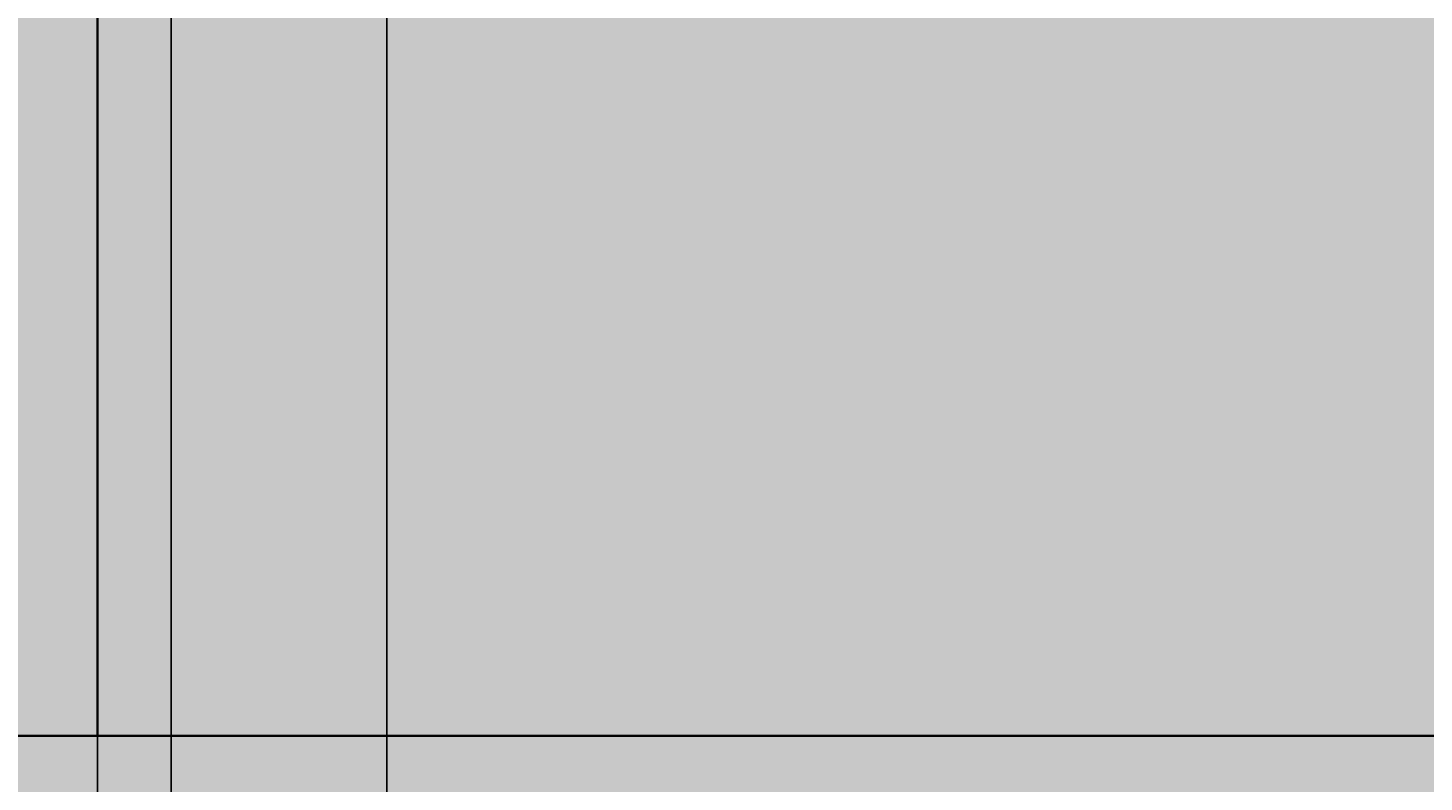
# Model space of a CAD drawing. Units: feet. Extents: x 2695 to 2912, y 795 to 1139.
# Tile 68 of 83: x 2769 to 2805, y 1062 to 1081. Entities that reach past the tile are written whole.
import ezdxf

# ---------------------------------------------------------------- set-up
doc = ezdxf.new("R2010")
doc.units = ezdxf.units.FT
for name, color, linetype, lineweight in [('A-ANNO-DIMS', 2, 'Continuous', 18), ('A-ELEV', 7, 'Continuous', 35), ('A-ELEV-PATT', 252, 'Continuous', 13)]:
    doc.layers.add(name, color=color, linetype=linetype, lineweight=lineweight)
doc.styles.get("Standard").update_dxf_attribs({"font": 'arial.ttf'})
doc.dimstyles.get("Standard").update_dxf_attribs({"dimtxt": 0.18, "dimasz": 0.18, "dimexe": 0.18, "dimexo": 0.0625, "dimgap": 0.09, "dimtad": 0, "dimtih": 1, "dimtoh": 1, "dimdec": 1, "dimzin": 0, "dimdsep": 46, "dimlunit": 3, "dimtxsty": 'Standard', "dimcen": 0.09, "dimadec": 0, "dimazin": 0, "dimtfac": 1, "dimtdec": 1, "dimtofl": 0, "dimtmove": 0, "dimatfit": 3, "dimfxl": 1, "dimtolj": 1, "dimtzin": 0, "dimarcsym": 0})

# ---------------------------------------------------------------- blocks, each defined once
blk = doc.blocks.new('*D8')
at = {"layer": 'A-ANNO-DIMS', "color": 0, "lineweight": -2, "transparency": 16777216}
for p, q in [((2715.885, 1050.373), (2715.885, 1138.886)), ((2716.065, 1138.706), (2742.866, 1138.706)), ((2770.456, 1138.706), (2743.655, 1138.706)), ((2770.636, 1122.993), (2770.636, 1138.886))]:
    blk.add_line(p, q, dxfattribs=at)
at = {"layer": 'A-ANNO-DIMS', "color": 0, "transparency": 16777216}
for points in [[(2716.065, 1138.736), (2716.065, 1138.676), (2715.885, 1138.706)], [(2770.456, 1138.736), (2770.456, 1138.676), (2770.636, 1138.706)]]:
    blk.add_solid(points, dxfattribs=at)
at = {"layer": 'Defpoints', "color": 0, "transparency": 16777216}
for p in [(2770.636, 1138.706), (2770.636, 1122.931), (2715.885, 1050.311)]:
    blk.add_point(p, dxfattribs=at)
at = {"layer": 'A-ANNO-DIMS', "color": 0, "transparency": 16777216, "insert": (2743.261, 1138.706), "char_height": 0.18, "attachment_point": 5}
blk.add_mtext('\\A1;54.75', dxfattribs=at)
blk = doc.blocks.new('*D9')
at = {"layer": 'A-ANNO-DIMS', "color": 0, "lineweight": -2, "transparency": 16777216}
for p, q in [((2770.636, 1122.993), (2770.636, 1138.886)), ((2770.816, 1138.706), (2773.942, 1138.706)), ((2777.854, 1138.706), (2774.728, 1138.706)), ((2778.034, 1020.886), (2778.034, 1138.886))]:
    blk.add_line(p, q, dxfattribs=at)
at = {"layer": 'A-ANNO-DIMS', "color": 0, "transparency": 16777216}
for points in [[(2770.816, 1138.736), (2770.816, 1138.676), (2770.636, 1138.706)], [(2777.854, 1138.736), (2777.854, 1138.676), (2778.034, 1138.706)]]:
    blk.add_solid(points, dxfattribs=at)
at = {"layer": 'Defpoints', "color": 0, "transparency": 16777216}
for p in [(2778.034, 1138.706), (2770.636, 1122.931), (2778.034, 1020.824)]:
    blk.add_point(p, dxfattribs=at)
at = {"layer": 'A-ANNO-DIMS', "color": 0, "transparency": 16777216, "insert": (2774.335, 1138.706), "char_height": 0.18, "attachment_point": 5}
blk.add_mtext('\\A1;7.398', dxfattribs=at)
blk = doc.blocks.new('*D10')
at = {"layer": 'A-ANNO-DIMS', "color": 0, "lineweight": -2, "transparency": 16777216}
for p, q in [((2778.034, 1020.886), (2778.034, 1138.886)), ((2778.214, 1138.706), (2810.411, 1138.706)), ((2843.395, 1138.706), (2811.198, 1138.706)), ((2843.575, 1020.886), (2843.575, 1138.886))]:
    blk.add_line(p, q, dxfattribs=at)
at = {"layer": 'A-ANNO-DIMS', "color": 0, "transparency": 16777216}
for points in [[(2778.214, 1138.736), (2778.214, 1138.676), (2778.034, 1138.706)], [(2843.395, 1138.736), (2843.395, 1138.676), (2843.575, 1138.706)]]:
    blk.add_solid(points, dxfattribs=at)
at = {"layer": 'Defpoints', "color": 0, "transparency": 16777216}
for p in [(2843.575, 1138.706), (2778.034, 1020.824), (2843.575, 1020.824)]:
    blk.add_point(p, dxfattribs=at)
at = {"layer": 'A-ANNO-DIMS', "color": 0, "transparency": 16777216, "insert": (2810.805, 1138.706), "char_height": 0.18, "attachment_point": 5}
blk.add_mtext('\\A1;65.54', dxfattribs=at)
blk = doc.blocks.new('*D48')
at = {"layer": 'A-ANNO-DIMS', "color": 0, "lineweight": -2, "transparency": 16777216}
for p, q in [((2770.636, 972.03), (2770.636, 1138.886)), ((2770.816, 1138.706), (2771.263, 1138.706)), ((2772.342, 1138.706), (2771.894, 1138.706)), ((2772.522, 972.03), (2772.522, 1138.886))]:
    blk.add_line(p, q, dxfattribs=at)
at = {"layer": 'A-ANNO-DIMS', "color": 0, "transparency": 16777216}
for points in [[(2770.816, 1138.736), (2770.816, 1138.676), (2770.636, 1138.706)], [(2772.342, 1138.736), (2772.342, 1138.676), (2772.522, 1138.706)]]:
    blk.add_solid(points, dxfattribs=at)
at = {"layer": 'Defpoints', "color": 0, "transparency": 16777216}
for p in [(2772.522, 1138.706), (2770.636, 971.967), (2772.522, 971.967)]:
    blk.add_point(p, dxfattribs=at)
at = {"layer": 'A-ANNO-DIMS', "color": 0, "transparency": 16777216, "insert": (2771.579, 1138.706), "char_height": 0.18, "attachment_point": 5}
blk.add_mtext('\\A1;1.89', dxfattribs=at)
blk = doc.blocks.new('*D49')
at = {"layer": 'A-ANNO-DIMS', "color": 0, "lineweight": -2, "transparency": 16777216}
for p, q in [((2772.522, 972.03), (2772.522, 1138.886)), ((2772.702, 1138.706), (2790.888, 1138.706)), ((2809.861, 1138.706), (2791.674, 1138.706)), ((2810.041, 972.03), (2810.041, 1138.886))]:
    blk.add_line(p, q, dxfattribs=at)
at = {"layer": 'A-ANNO-DIMS', "color": 0, "transparency": 16777216}
for points in [[(2772.702, 1138.736), (2772.702, 1138.676), (2772.522, 1138.706)], [(2809.861, 1138.736), (2809.861, 1138.676), (2810.041, 1138.706)]]:
    blk.add_solid(points, dxfattribs=at)
at = {"layer": 'Defpoints', "color": 0, "transparency": 16777216}
for p in [(2810.041, 1138.706), (2772.522, 971.967), (2810.041, 971.967)]:
    blk.add_point(p, dxfattribs=at)
at = {"layer": 'A-ANNO-DIMS', "color": 0, "transparency": 16777216, "insert": (2791.281, 1138.706), "char_height": 0.18, "attachment_point": 5}
blk.add_mtext('\\A1;37.52', dxfattribs=at)

msp = doc.modelspace()

# ---------------------------------------------------------------- hatches: boundary and pattern name
at = {"layer": 'A-ELEV-PATT'}
h = msp.add_hatch(color=256, dxfattribs=at)
h.set_gradient(color1=(255, 255, 255), tint=1)
h.paths.add_polyline_path([(2770.6361, 1122.9306), (2710.6361, 1122.9306), (2710.6361, 1118.4096), (2770.6361, 1118.4096)])
h.paths.add_polyline_path([(2890.6361, 1107.8588), (2770.6361, 1107.8588), (2770.6361, 1103.3378), (2890.6361, 1103.3378)])
h.paths.add_polyline_path([(2890.6361, 1062.9306), (2710.6361, 1062.9306), (2710.6361, 1056.9306), (2710.6361, 936.9306), (2710.6361, 924.3105), (2716.5358, 924.3105), (2890.6361, 924.3105), (2890.6361, 936.9306), (2715.8852, 936.9306), (2715.8852, 1050.3105), (2890.6361, 1050.3105)])
h.paths.add_polyline_path([(2716.5358, 924.3105), (2710.6361, 924.3105), (2710.6361, 810.9306), (2716.5358, 810.9306)])
h = msp.add_hatch(color=256, dxfattribs=at)
h.set_gradient(color1=(147, 149, 152), color2=(147, 149, 152), tint=1)
h.paths.add_polyline_path([(2770.6361, 1118.4096), (2710.6361, 1118.4096), (2710.6361, 1062.9306), (2770.6361, 1062.9306)])
h.paths.add_polyline_path([(2890.6361, 1103.3378), (2770.6361, 1103.3378), (2770.6361, 1062.9306), (2890.6361, 1062.9306)])
h.paths.add_polyline_path([(2730.7081, 1048.1052), (2755.1125, 1048.1052), (2755.1125, 936.9306), (2770.6361, 936.9306), (2770.6361, 1050.3105), (2715.8852, 1050.3105), (2715.8852, 936.9306), (2730.7081, 936.9306)])
h.paths.add_polyline_path([(2890.6361, 1050.3105), (2770.6361, 1050.3105), (2770.6361, 971.9673), (2778.0341, 971.9673), (2778.0341, 1020.8235), (2843.575, 1020.8235), (2843.575, 971.9673), (2890.6361, 971.9673)])
h.paths.add_polyline_path([(2888.1882, 970.7156), (2843.575, 970.7156), (2843.575, 964.8267), (2888.1882, 964.8267)])
h.paths.add_polyline_path([(2888.1882, 964.1328), (2843.575, 964.1328), (2843.575, 956.614), (2888.1882, 956.614)])
h.paths.add_polyline_path([(2888.1882, 955.9202), (2843.575, 955.9202), (2843.575, 949.2892), (2888.1882, 949.2892)])
h.paths.add_polyline_path([(2888.1882, 948.5954), (2843.575, 948.5954), (2843.575, 941.3507), (2888.1882, 941.3507)])
h.paths.add_polyline_path([(2888.1882, 940.6569), (2843.575, 940.6569), (2843.575, 936.9306), (2888.1882, 936.9306)])
h.paths.add_polyline_path([(2890.6361, 970.7156), (2888.9368, 970.7156), (2888.9368, 964.8267), (2890.6361, 964.8267)])
h.paths.add_polyline_path([(2890.6361, 964.1328), (2888.9368, 964.1328), (2888.9368, 956.614), (2890.6361, 956.614)])
h.paths.add_polyline_path([(2890.6361, 955.9202), (2888.9368, 955.9202), (2888.9368, 949.2892), (2890.6361, 949.2892)])
h.paths.add_polyline_path([(2890.6361, 940.6569), (2888.9368, 940.6569), (2888.9368, 936.9306), (2890.6361, 936.9306)])
h.paths.add_polyline_path([(2890.6361, 948.5954), (2888.9368, 948.5954), (2888.9368, 941.3507), (2890.6361, 941.3507)])
h.paths.add_polyline_path([(2772.5216, 970.7156), (2770.6361, 970.7156), (2770.6361, 964.8267), (2772.5216, 964.8267)])
h.paths.add_polyline_path([(2772.5216, 964.1328), (2770.6361, 964.1328), (2770.6361, 956.614), (2772.5216, 956.614)])
h.paths.add_polyline_path([(2772.5216, 955.9202), (2770.6361, 955.9202), (2770.6361, 949.2892), (2772.5216, 949.2892)])
h.paths.add_polyline_path([(2772.5216, 948.5954), (2770.6361, 948.5954), (2770.6361, 941.3507), (2772.5216, 941.3507)])
h.paths.add_polyline_path([(2772.5216, 940.6569), (2770.6361, 940.6569), (2770.6361, 936.9306), (2772.5216, 936.9306)])
h.paths.add_polyline_path([(2778.0341, 940.6569), (2773.2702, 940.6569), (2773.2702, 936.9306), (2778.0341, 936.9306)])
h.paths.add_polyline_path([(2778.0341, 970.7156), (2773.2702, 970.7156), (2773.2702, 964.8267), (2778.0341, 964.8267)])
h.paths.add_polyline_path([(2778.0341, 964.1328), (2773.2702, 964.1328), (2773.2702, 956.614), (2778.0341, 956.614)])
h.paths.add_polyline_path([(2778.0341, 955.9202), (2773.2702, 955.9202), (2773.2702, 949.2892), (2778.0341, 949.2892)])
h.paths.add_polyline_path([(2778.0341, 948.5954), (2773.2702, 948.5954), (2773.2702, 941.3507), (2778.0341, 941.3507)])
h.paths.add_polyline_path([(2810.0407, 940.6569), (2780.0341, 940.6569), (2780.0341, 936.9306), (2810.0407, 936.9306)])
h.paths.add_polyline_path([(2890.6361, 924.3105), (2770.6361, 924.3105), (2770.6361, 810.9306), (2773.5029, 810.9306), (2773.5029, 905.5143), (2805.9398, 905.5143), (2838.3767, 905.5143), (2838.3767, 810.9306), (2890.6361, 810.9306)])
h = msp.add_hatch(color=256, dxfattribs=at)
h.set_gradient(color1=(199, 200, 202), color2=(213, 227, 240), centered=1)
h.paths.add_polyline_path([(2890.6361, 1103.3378), (2770.6361, 1103.3378), (2770.6361, 1062.9306), (2890.6361, 1062.9306)])

# ---------------------------------------------------------------- linework, layer by layer
at = {"layer": 'A-ELEV'}
for p, q in [((2770.6361, 1122.9306), (2770.6361, 1062.9306)), ((2710.6361, 1062.9306), (2890.6361, 1062.9306)), ((2710.6361, 1062.9306), (2895.4694, 1062.9306))]:
    msp.add_line(p, q, dxfattribs=at)

# ---------------------------------------------------------------- dimensions: what is measured, and where the dimension line sits
at = {"layer": 'A-ANNO-DIMS'}
for base, p1, p2, override, picture, middle in [((2770.6361, 1138.7056), (2715.8852, 1050.3105), (2770.6361, 1122.9306), {"dimdec": 2, "dimlfac": 1, "dimrnd": 0, "dimzin": 0, "dimdsep": 46, "dimlunit": 2}, '*D8', (2743.2606, 1138.7056)), ((2778.0341, 1138.7056), (2770.6361, 1122.9306), (2778.0341, 1020.8235), {"dimdec": 3, "dimlfac": 1, "dimrnd": 0, "dimzin": 0, "dimdsep": 46, "dimlunit": 2}, '*D9', (2774.3351, 1138.7056)), ((2772.5216, 1138.7056), (2770.6361, 971.9673), (2772.5216, 971.9673), {"dimdec": 2, "dimlfac": 1, "dimrnd": 0, "dimzin": 0, "dimdsep": 46, "dimlunit": 2}, '*D48', (2771.5788, 1138.7056)), ((2810.0407, 1138.7056), (2772.5216, 971.9673), (2810.0407, 971.9673), {"dimdec": 2, "dimlfac": 1, "dimrnd": 0, "dimzin": 0, "dimdsep": 46, "dimlunit": 2}, '*D49', (2791.2811, 1138.7056)), ((2843.575, 1138.7056), (2778.0341, 1020.8235), (2843.575, 1020.8235), {"dimdec": 2, "dimlfac": 1, "dimrnd": 0, "dimzin": 0, "dimdsep": 46, "dimlunit": 2}, '*D10', (2810.8045, 1138.7056))]:
    dim = msp.add_linear_dim(base=base, p1=p1, p2=p2, dimstyle='Standard', override=override, dxfattribs=at)
    dim.commit()
    dim.dimension.update_dxf_attribs({"geometry": picture, "text_midpoint": middle})

doc.saveas('drawing.dxf')
